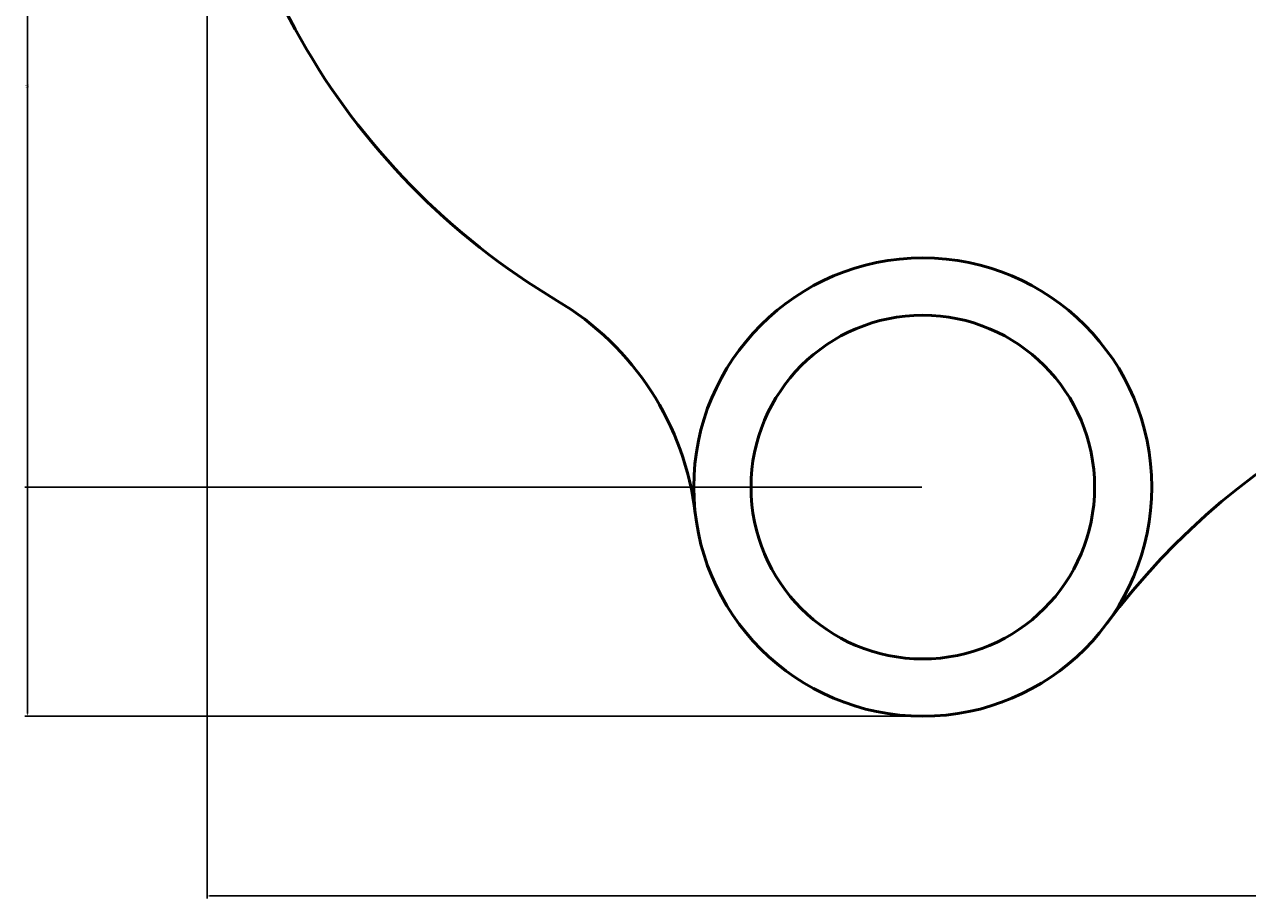
# Model space of a CAD drawing. Units: inches. Extents: x -307 to -76, y 16 to 196.
# Tile 1 of 7: x -307 to -222, y 16 to 77. Entities that reach past the tile are written whole.
import ezdxf

# ---------------------------------------------------------------- set-up
doc = ezdxf.new("R2010")
doc.units = ezdxf.units.IN
doc.header["$MEASUREMENT"] = 0
doc.layers.add('M-DIMS', color=2, linetype='Continuous', lineweight=18)
doc.layers.add('M-OUTL', color=7, linetype='Continuous', lineweight=50)
doc.styles.get("Standard").update_dxf_attribs({"font": 'arial.ttf'})
doc.dimstyles.get("Standard").update_dxf_attribs({"dimtxt": 0.18, "dimasz": 0.18, "dimexe": 0.18, "dimexo": 0.0625, "dimgap": 0.09, "dimtad": 0, "dimtih": 1, "dimtoh": 1, "dimdec": 4, "dimzin": 0, "dimdsep": 46, "dimtxsty": 'Standard', "dimcen": 0.09, "dimadec": 0, "dimazin": 0, "dimtfac": 1, "dimtdec": 4, "dimtofl": 0, "dimtmove": 0, "dimatfit": 3, "dimfxl": 1, "dimtolj": 1, "dimtzin": 0, "dimarcsym": 0})

# ---------------------------------------------------------------- blocks, each defined once
blk = doc.blocks.new('BORE-D24-RIM-D32')
for radius in [16, 12]:
    blk.add_circle((16, 16), radius)
blk = doc.blocks.new('*D2')
at = {"layer": 'Defpoints', "color": 0, "transparency": 16777216}
for p in [(-294.39, 101), (-88.39, 101), (-88.39, 16.45)]:
    blk.add_point(p, dxfattribs=at)
at = {"layer": 'M-DIMS', "color": 0, "lineweight": -2, "transparency": 16777216}
for p, q in [((-294.39, 100.938), (-294.39, 16.27)), ((-88.39, 100.938), (-88.39, 16.27)), ((-294.21, 16.45), (-191.68, 16.45)), ((-88.57, 16.45), (-191.099, 16.45))]:
    blk.add_line(p, q, dxfattribs=at)
at = {"layer": 'M-DIMS', "color": 0, "transparency": 16777216}
for points in [[(-294.21, 16.48), (-294.21, 16.42), (-294.39, 16.45)], [(-88.57, 16.48), (-88.57, 16.42), (-88.39, 16.45)]]:
    blk.add_solid(points, dxfattribs=at)
at = {"layer": 'M-DIMS', "color": 0, "transparency": 16777216, "insert": (-191.39, 16.45), "char_height": 0.18, "attachment_point": 5}
blk.add_mtext('\\A1;206', dxfattribs=at)
blk = doc.blocks.new('*D3')
at = {"layer": 'Defpoints', "color": 0, "transparency": 16777216}
for p in [(-306.94, 173), (-244.39, 173), (-244.39, 29)]:
    blk.add_point(p, dxfattribs=at)
at = {"layer": 'M-DIMS', "color": 0, "lineweight": -2, "transparency": 16777216}
for p, q in [((-244.452, 173), (-307.12, 173)), ((-306.94, 172.82), (-306.94, 101.18)), ((-306.94, 29.18), (-306.94, 100.82)), ((-244.452, 29), (-307.12, 29))]:
    blk.add_line(p, q, dxfattribs=at)
at = {"layer": 'M-DIMS', "color": 0, "transparency": 16777216}
for points in [[(-306.97, 172.82), (-306.91, 172.82), (-306.94, 173)], [(-306.97, 29.18), (-306.91, 29.18), (-306.94, 29)]]:
    blk.add_solid(points, dxfattribs=at)
at = {"layer": 'M-DIMS', "color": 0, "transparency": 16777216, "insert": (-306.94, 101), "char_height": 0.18, "attachment_point": 5}
blk.add_mtext('\\A1;144', dxfattribs=at)
blk = doc.blocks.new('*D6')
at = {"layer": 'Defpoints', "color": 0, "transparency": 16777216}
for p in [(-306.94, 101), (-244.39, 101), (-244.39, 45)]:
    blk.add_point(p, dxfattribs=at)
at = {"layer": 'M-DIMS', "color": 0, "lineweight": -2, "transparency": 16777216}
for p, q in [((-244.452, 101), (-307.12, 101)), ((-306.94, 100.82), (-306.94, 73.182)), ((-306.94, 45.18), (-306.94, 72.818)), ((-244.452, 45), (-307.12, 45))]:
    blk.add_line(p, q, dxfattribs=at)
at = {"layer": 'M-DIMS', "color": 0, "transparency": 16777216}
for points in [[(-306.97, 100.82), (-306.91, 100.82), (-306.94, 101)], [(-306.97, 45.18), (-306.91, 45.18), (-306.94, 45)]]:
    blk.add_solid(points, dxfattribs=at)
at = {"layer": 'M-DIMS', "color": 0, "transparency": 16777216, "insert": (-306.94, 73), "char_height": 0.18, "attachment_point": 5}
blk.add_mtext('\\A1;56', dxfattribs=at)

msp = doc.modelspace()

# ---------------------------------------------------------------- linework, layer by layer
at = {"layer": 'M-OUTL'}
for centre, radius, start, end in [((-244.39, 101), 50, 120.71777, 239.28223), ((-280.146, 40.821), 20, 6.66543, 59.28223), ((-191.39, 5.668), 50, 36.57954, 143.42046)]:
    msp.add_arc(centre, radius, start, end, dxfattribs=at)

# ---------------------------------------------------------------- block references
msp.add_blockref('BORE-D24-RIM-D32', (-260.39, 29), dxfattribs=at)

# ---------------------------------------------------------------- dimensions: what is measured, and where the dimension line sits
at = {"layer": 'M-DIMS'}
for base, p1, p2, picture, middle in [((-306.94, 173), (-244.39, 29), (-244.39, 173), '*D3', (-306.94, 101)), ((-306.94, 101), (-244.39, 45), (-244.39, 101), '*D6', (-306.94, 73))]:
    dim = msp.add_linear_dim(base=base, p1=p1, p2=p2, angle=90, dimstyle='Standard', override={"dimdec": 0, "dimlfac": 1, "dimrnd": 0, "dimzin": 0, "dimdsep": 46, "dimlunit": 2}, dxfattribs=at)
    dim.commit()
    dim.dimension.update_dxf_attribs({"geometry": picture, "text_midpoint": middle})
dim = msp.add_linear_dim(base=(-88.39, 16.45), p1=(-294.39, 101), p2=(-88.39, 101), dimstyle='Standard', override={"dimdec": 0, "dimlfac": 1, "dimrnd": 0, "dimzin": 0, "dimdsep": 46, "dimlunit": 2}, dxfattribs=at)
dim.commit()
dim.dimension.update_dxf_attribs({"geometry": '*D2', "text_midpoint": (-191.39, 16.45)})

doc.saveas('drawing.dxf')
